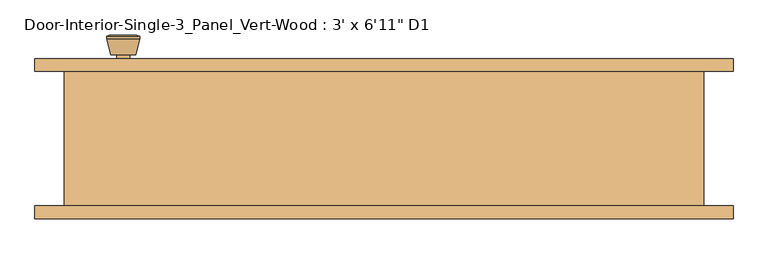
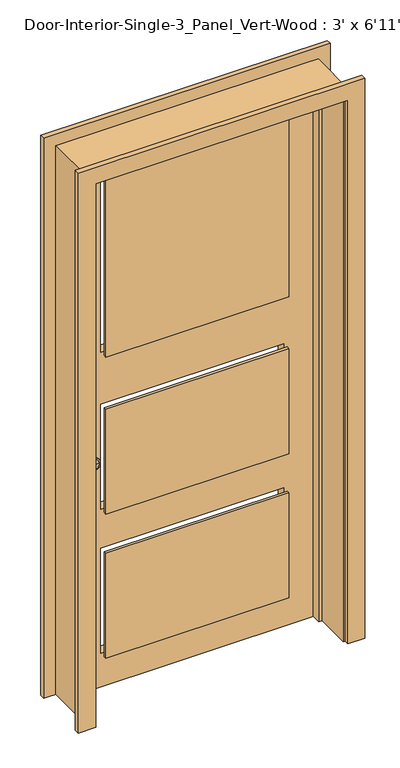
"""IFC4 building model written with IfcOpenShell, lengths in millimetres: door geometry."""

from ifc_helpers import new_model, si_unit, point, frame, frame_2d, origin, place, context, project, spatial, polyline, circle_curve, trimmed, segment, composite_curve, outline, extrude, faceted_brep, source, transform, mapped, element, save
from ifc_brep_helpers import plane_surface, cylinder_surface, revolved_surface, advanced_brep


def door_721a2355(model_context):
    return source(origin(), model_context, "Body", "SolidModel", [
        advanced_brep(
        [(-393.7, 57.5, 914.4), (-383.7, 57.5, 914.4), (-403.7, 57.5, 914.4), (-373.2241324, 8.5, 914.4), (-393.7, 8.5, 914.4), (-414.1758676, 8.5, 914.4), (-368.7, 10.3278681, 914.4), (-418.7, 10.3278681, 914.4), (-368.7, 13.7915463, 914.4), (-418.7, 13.7915463, 914.4), (-375.063764, 38.5, 914.4), (-412.336236, 38.5, 914.4), (-383.7, 38.5, 914.4), (-403.7, 38.5, 914.4)],
        [
            (0, 1),
            (1, 2, circle_curve(frame((-393.7, 57.5, 914.4), z_axis=(0.0, 1.0, 0.0), x_axis=(-1.0, 0.0, 0.0)), 10.0)),
            (2, 0),
            (2, 1, circle_curve(frame((-393.7, 57.5, 914.4), z_axis=(0.0, 1.0, 0.0), x_axis=(-1.0, 0.0, 0.0)), 10.0)),
            (3, 4),
            (4, 5),
            (5, 3, circle_curve(frame((-393.7, 8.5, 914.4), z_axis=(0.0, -1.0, 0.0), x_axis=(-1.0, 0.0, 0.0)), 20.4758676)),
            (3, 5, circle_curve(frame((-393.7, 8.5, 914.4), z_axis=(0.0, -1.0, 0.0), x_axis=(-1.0, 0.0, 0.0)), 20.4758676)),
            (6, 3),
            (5, 7),
            (7, 6, circle_curve(frame((-393.7, 10.3278681, 914.4), z_axis=(0.0, -1.0, 0.0), x_axis=(-1.0, 0.0, 0.0)), 25.0)),
            (6, 7, circle_curve(frame((-393.7, 10.3278681, 914.4), z_axis=(0.0, -1.0, 0.0), x_axis=(-1.0, 0.0, 0.0)), 25.0)),
            (8, 6),
            (7, 9),
            (9, 8, circle_curve(frame((-393.7, 13.7915463, 914.4), z_axis=(0.0, -1.0, 0.0), x_axis=(-1.0, 0.0, 0.0)), 25.0)),
            (8, 9, circle_curve(frame((-393.7, 13.7915463, 914.4), z_axis=(0.0, -1.0, 0.0), x_axis=(-1.0, 0.0, 0.0)), 25.0)),
            (10, 8),
            (9, 11),
            (11, 10, circle_curve(frame((-393.7, 38.5, 914.4), z_axis=(0.0, -1.0, 0.0), x_axis=(-1.0, 0.0, 0.0)), 18.636236)),
            (10, 11, circle_curve(frame((-393.7, 38.5, 914.4), z_axis=(0.0, -1.0, 0.0), x_axis=(-1.0, 0.0, 0.0)), 18.636236)),
            (12, 10),
            (11, 13),
            (13, 12, circle_curve(frame((-393.7, 38.5, 914.4), z_axis=(0.0, -1.0, 0.0), x_axis=(-1.0, 0.0, 0.0)), 10.0)),
            (12, 13, circle_curve(frame((-393.7, 38.5, 914.4), z_axis=(0.0, -1.0, 0.0), x_axis=(-1.0, 0.0, 0.0)), 10.0)),
            (1, 12),
            (13, 2),
        ],
        [
            plane_surface(frame((-393.7, 57.5, 914.4), z_axis=(0.0, 1.0, 0.0), x_axis=(-1.0, 0.0, 0.0))),
            plane_surface(frame((-393.7, 8.5, 914.4), z_axis=(0.0, -1.0, 0.0), x_axis=(-1.0, 0.0, 0.0))),
            revolved_surface(polyline([(-414.1758676, 8.5, 914.4), (-418.7, 10.3278681, 914.4)]), (-393.7, 57.5, 914.4), (0.0, 1.0, 0.0)),
            cylinder_surface(frame((-393.7, 57.5, 914.4), z_axis=(0.0, 1.0, 0.0), x_axis=(-1.0, 0.0, 0.0)), 25.0),
            revolved_surface(polyline([(-418.7, 13.7915463, 914.4), (-412.336236, 38.5, 914.4)]), (-393.7, 57.5, 914.4), (0.0, 1.0, 0.0)),
            plane_surface(frame((-393.7, 38.5, 914.4), z_axis=(0.0, 1.0, 0.0), x_axis=(-1.0, 0.0, 0.0))),
            cylinder_surface(frame((-393.7, 57.5, 914.4), z_axis=(0.0, 1.0, 0.0), x_axis=(-1.0, 0.0, 0.0)), 10.0),
        ],
        [
            (0, [[1, 2, 3]]),
            (0, [[-3, 4, -1]]),
            (1, [[5, 6, 7]]),
            (1, [[-6, -5, 8]]),
            (2, [[9, -7, 10, 11]]),
            (2, [[-10, -8, -9, 12]]),
            (3, [[13, -11, 14, 15]]),
            (3, [[-14, -12, -13, 16]]),
            (4, [[17, -15, 18, 19]]),
            (4, [[-18, -16, -17, 20]]),
            (5, [[21, -19, 22, 23]]),
            (5, [[-22, -20, -21, 24]]),
            (6, [[25, -23, 26, -2]]),
            (6, [[-26, -24, -25, -4]]),
        ],
    ),
        extrude(outline(composite_curve([segment(trimmed(circle_curve(frame_2d((914.4, -393.7)), 30.0), [point((914.4, -423.7))], [point((914.4, -363.7))], False, "CARTESIAN"), True, "CONTINUOUS"), segment(trimmed(circle_curve(frame_2d((914.4, -393.7)), 30.0), [point((914.4, -363.7))], [point((914.4, -423.7))], False, "CARTESIAN"), True, "CONTINUOUS")], self_intersect=False)), frame((0.0, 57.5, 0.0), z_axis=(0.0, 1.0, 0.0), x_axis=(0.0, 0.0, 1.0)), (0.0, 0.0, 1.0), 6.0),
        advanced_brep(
        [(-393.7, 104.425, 914.4), (-403.7, 104.425, 914.4), (-383.7, 104.425, 914.4), (-373.2241324, 153.425, 914.4), (-414.1758676, 153.425, 914.4), (-393.7, 153.425, 914.4), (-368.7, 151.5971319, 914.4), (-418.7, 151.5971319, 914.4), (-368.7, 148.1334537, 914.4), (-418.7, 148.1334537, 914.4), (-375.063764, 123.425, 914.4), (-412.336236, 123.425, 914.4), (-383.7, 123.425, 914.4), (-403.7, 123.425, 914.4)],
        [
            (0, 1),
            (1, 2, circle_curve(frame((-393.7, 104.425, 914.4), z_axis=(0.0, -1.0, 0.0), x_axis=(-1.0, 0.0, 0.0)), 10.0)),
            (2, 0),
            (2, 1, circle_curve(frame((-393.7, 104.425, 914.4), z_axis=(0.0, -1.0, 0.0), x_axis=(-1.0, 0.0, 0.0)), 10.0)),
            (3, 4, circle_curve(frame((-393.7, 153.425, 914.4), z_axis=(0.0, 1.0, 0.0), x_axis=(-1.0, 0.0, 0.0)), 20.4758676)),
            (4, 5),
            (5, 3),
            (4, 3, circle_curve(frame((-393.7, 153.425, 914.4), z_axis=(0.0, 1.0, 0.0), x_axis=(-1.0, 0.0, 0.0)), 20.4758676)),
            (6, 7, circle_curve(frame((-393.7, 151.5971319, 914.4), z_axis=(0.0, 1.0, 0.0), x_axis=(-1.0, 0.0, 0.0)), 25.0)),
            (7, 4),
            (3, 6),
            (7, 6, circle_curve(frame((-393.7, 151.5971319, 914.4), z_axis=(0.0, 1.0, 0.0), x_axis=(-1.0, 0.0, 0.0)), 25.0)),
            (8, 9, circle_curve(frame((-393.7, 148.1334537, 914.4), z_axis=(0.0, 1.0, 0.0), x_axis=(-1.0, 0.0, 0.0)), 25.0)),
            (9, 7),
            (6, 8),
            (9, 8, circle_curve(frame((-393.7, 148.1334537, 914.4), z_axis=(0.0, 1.0, 0.0), x_axis=(-1.0, 0.0, 0.0)), 25.0)),
            (10, 11, circle_curve(frame((-393.7, 123.425, 914.4), z_axis=(0.0, 1.0, 0.0), x_axis=(-1.0, 0.0, 0.0)), 18.636236)),
            (11, 9),
            (8, 10),
            (11, 10, circle_curve(frame((-393.7, 123.425, 914.4), z_axis=(0.0, 1.0, 0.0), x_axis=(-1.0, 0.0, 0.0)), 18.636236)),
            (12, 13, circle_curve(frame((-393.7, 123.425, 914.4), z_axis=(0.0, 1.0, 0.0), x_axis=(-1.0, 0.0, 0.0)), 10.0)),
            (13, 11),
            (10, 12),
            (13, 12, circle_curve(frame((-393.7, 123.425, 914.4), z_axis=(0.0, 1.0, 0.0), x_axis=(-1.0, 0.0, 0.0)), 10.0)),
            (1, 13),
            (12, 2),
        ],
        [
            plane_surface(frame((-393.7, 104.425, 914.4), z_axis=(0.0, -1.0, 0.0), x_axis=(-1.0, 0.0, 0.0))),
            plane_surface(frame((-393.7, 153.425, 914.4), z_axis=(0.0, 1.0, 0.0), x_axis=(-1.0, 0.0, 0.0))),
            revolved_surface(polyline([(-414.1758676, 153.425, 914.4), (-418.7, 151.5971319, 914.4)]), (-393.7, 104.425, 914.4), (0.0, -1.0, 0.0)),
            cylinder_surface(frame((-393.7, 104.425, 914.4), z_axis=(0.0, -1.0, 0.0), x_axis=(-1.0, 0.0, 0.0)), 25.0),
            revolved_surface(polyline([(-418.7, 148.1334537, 914.4), (-412.336236, 123.425, 914.4)]), (-393.7, 104.425, 914.4), (0.0, -1.0, 0.0)),
            plane_surface(frame((-393.7, 123.425, 914.4), z_axis=(0.0, -1.0, 0.0), x_axis=(-1.0, 0.0, 0.0))),
            cylinder_surface(frame((-393.7, 104.425, 914.4), z_axis=(0.0, -1.0, 0.0), x_axis=(-1.0, 0.0, 0.0)), 10.0),
        ],
        [
            (0, [[1, 2, 3]]),
            (0, [[-3, 4, -1]]),
            (1, [[5, 6, 7]]),
            (1, [[8, -7, -6]]),
            (2, [[9, 10, -5, 11]]),
            (2, [[12, -11, -8, -10]]),
            (3, [[13, 14, -9, 15]]),
            (3, [[16, -15, -12, -14]]),
            (4, [[17, 18, -13, 19]]),
            (4, [[20, -19, -16, -18]]),
            (5, [[21, 22, -17, 23]]),
            (5, [[24, -23, -20, -22]]),
            (6, [[-2, 25, -21, 26]]),
            (6, [[-4, -26, -24, -25]]),
        ],
    ),
        extrude(outline(composite_curve([segment(trimmed(circle_curve(frame_2d((914.4, -393.7)), 30.0), [point((914.4, -423.7))], [point((914.4, -363.7))], False, "CARTESIAN"), True, "CONTINUOUS"), segment(trimmed(circle_curve(frame_2d((914.4, -393.7)), 30.0), [point((914.4, -363.7))], [point((914.4, -423.7))], False, "CARTESIAN"), True, "CONTINUOUS")], self_intersect=False)), frame((0.0, 98.425, 0.0), z_axis=(0.0, 1.0, 0.0), x_axis=(0.0, 0.0, 1.0)), (0.0, 0.0, 1.0), 6.0),
        faceted_brep([(482.6, 98.425, 0.0), (482.6, -104.775, 0.0), (457.2, -104.775, 0.0), (457.2, 28.575, 0.0), (444.5, 28.575, 0.0), (444.5, 63.5, 0.0), (457.2, 63.5, 0.0), (457.2, 98.425, 0.0), (482.6, 98.425, 2133.6), (482.6, -104.775, 2133.6), (-482.6, -104.775, 2133.6), (-482.6, -104.775, 0.0), (-457.2, -104.775, 0.0), (-457.2, -104.775, 2108.2), (457.2, -104.775, 2108.2), (457.2, 28.575, 2108.2), (-457.2, 28.575, 2108.2), (-457.2, 28.575, 0.0), (-444.5, 28.575, 0.0), (-444.5, 28.575, 2095.5), (444.5, 28.575, 2095.5), (444.5, 63.5, 2095.5), (-444.5, 63.5, 2095.5), (-444.5, 63.5, 0.0), (-457.2, 63.5, 0.0), (-457.2, 63.5, 2108.2), (457.2, 63.5, 2108.2), (457.2, 98.425, 2108.2), (-457.2, 98.425, 2108.2), (-457.2, 98.425, 0.0), (-482.6, 98.425, 0.0), (-482.6, 98.425, 2133.6)], [[[0, 1, 2, 3, 4, 5, 6, 7]], [[1, 0, 8, 9]], [[2, 1, 9, 10, 11, 12, 13, 14]], [[3, 2, 14, 15]], [[4, 3, 15, 16, 17, 18, 19, 20]], [[5, 4, 20, 21]], [[6, 5, 21, 22, 23, 24, 25, 26]], [[7, 6, 26, 27]], [[0, 7, 27, 28, 29, 30, 31, 8]], [[9, 8, 31, 10]], [[15, 14, 13, 16]], [[21, 20, 19, 22]], [[27, 26, 25, 28]], [[30, 29, 24, 23, 18, 17, 12, 11]], [[10, 31, 30, 11]], [[16, 13, 12, 17]], [[22, 19, 18, 23]], [[28, 25, 24, 29]]]),
        extrude(outline(polyline([(2108.2, -457.2), (0.0, -457.2), (0.0, 457.2), (2108.2, 457.2), (2108.2, -457.2)]), holes=[polyline([(1989.1375, -336.55), (1989.1375, 336.55), (1301.75, 336.55), (1301.75, -336.55), (1989.1375, -336.55)]), polyline([(538.1625, -336.55), (538.1625, 336.55), (130.175, 336.55), (130.175, -336.55), (538.1625, -336.55)]), polyline([(1098.55, -336.55), (1098.55, 336.55), (690.5625, 336.55), (690.5625, -336.55), (1098.55, -336.55)])]), frame((0.0, 63.5, 0.0), z_axis=(0.0, 1.0, 0.0), x_axis=(0.0, 0.0, 1.0)), (0.0, 0.0, 1.0), 34.925),
        extrude(outline(polyline([(336.55, 30.6916667), (-336.55, 30.6916667), (-336.55, 42.3333333), (336.55, 42.3333333), (336.55, 30.6916667)])), frame((0.0, 0.0, 1301.75), z_axis=(0.0, 0.0, 1.0), x_axis=(1.0, 0.0, 0.0)), (0.0, 0.0, 1.0), 687.3875),
        extrude(outline(polyline([(336.55, 30.6916667), (-336.55, 30.6916667), (-336.55, 42.3333333), (336.55, 42.3333333), (336.55, 30.6916667)])), frame((0.0, 0.0, 130.175), z_axis=(0.0, 0.0, 1.0), x_axis=(1.0, 0.0, 0.0)), (0.0, 0.0, 1.0), 407.9875),
        extrude(outline(polyline([(336.55, 30.6916667), (-336.55, 30.6916667), (-336.55, 42.3333333), (336.55, 42.3333333), (336.55, 30.6916667)])), frame((0.0, 0.0, 690.5625), z_axis=(0.0, 0.0, 1.0), x_axis=(1.0, 0.0, 0.0)), (0.0, 0.0, 1.0), 407.9875),
        extrude(outline(polyline([(0.0, 463.55), (0.0, 527.05), (2178.05, 527.05), (2178.05, -527.05), (0.0, -527.05), (0.0, -463.55), (2114.55, -463.55), (2114.55, 463.55), (0.0, 463.55)])), frame((0.0, 98.425, 0.0), z_axis=(0.0, 1.0, 0.0), x_axis=(0.0, 0.0, 1.0)), (0.0, 0.0, 1.0), 19.05),
        extrude(outline(polyline([(0.0, 463.55), (0.0, 527.05), (2178.05, 527.05), (2178.05, -527.05), (0.0, -527.05), (0.0, -463.55), (2114.55, -463.55), (2114.55, 463.55), (0.0, 463.55)])), frame((0.0, -123.825, 0.0), z_axis=(0.0, 1.0, 0.0), x_axis=(0.0, 0.0, 1.0)), (0.0, 0.0, 1.0), 19.05),
    ])


if __name__ == "__main__":
    model = new_model("IFC4")
    model_context = context("Model", 3, world=origin())
    ifc_project = project(units=[si_unit("LENGTHUNIT", "METRE", prefix="MILLI")], contexts=[model_context])
    site = spatial("IfcSite", under=ifc_project)
    building = spatial("IfcBuilding", under=site)
    placement = place(None, origin())
    door_shape = door_721a2355(model_context)
    element("IfcDoor", 1, ObjectType="Door-Interior-Single-3_Panel_Vert-Wood : 3' x 6'11\" D1", at=placement, inside=building, context=model_context, shape_type="MappedRepresentation", body=[
        mapped(door_shape, transform((0.0, 0.0, 0.0), x_axis=(1.0, 0.0, 0.0), y_axis=(0.0, 1.0, 0.0), z_axis=(0.0, 0.0, 1.0))),
    ])
    save(model, "model.ifc")

# Revit data of these elements
# Type "Door-Interior-Single-3_Panel_Vert-Wood : 3' x 6'11\" D1"
#   Type Mark = "9"
#   Analytic Construction = "Wooden"
#   Top Rail = 0' - 4 11/16"
#   Thickness = 0' - 1 3/8"
#   Thermal Resistance (R) = 2.5876 (h·ft²·°F)/BTU
#   Swing Angle [instance default] = 90.00°
#   Stiles = 0' - 4 3/4"
#   Rough Width = 3' - 2"
#   Rough Height = 7' - 0"
#   Intermediate Rail = 0' - 4 1/2"
#   Height = 6' - 11"
#   Width = 3' - 0"
#   Heat Transfer Coefficient (U) = 0.3865 BTU/(h·ft²·°F)
#   Bottom Rail = 0' - 9 1/8"
#   Define Thermal Properties by = 1
#   Trim Material = Cherry
#   Panel Material = Cherry
#   Frame Material = Cherry
#   Door Handle Material = Aluminum
#   Visual Light Transmittance = 0
#   Solar Heat Gain Coefficient = 0
#   Wall Closure = (empty or 0)
#   Function = (empty or 0)
# Element 1 (IfcDoor, "Door-Interior-Single-3_Panel_Vert-Wood : 3' x 6'11\" D1")
#   Materials on its faces: "Cherry", "Aluminum"
# Materials
#   "Cherry": class "Wood", colour RGB 226 177 128, transparency 0, Description = "Prunus Serotina", Cost = 0
#   "Aluminum": class "Metal", colour RGB 247 247 247, transparency 0, Description = "Aluminum 6061", Cost = 0
